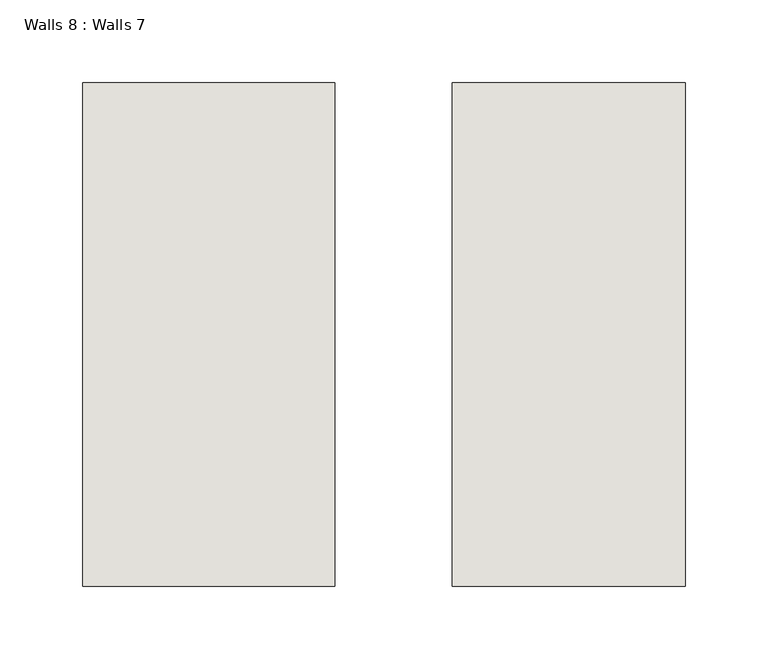
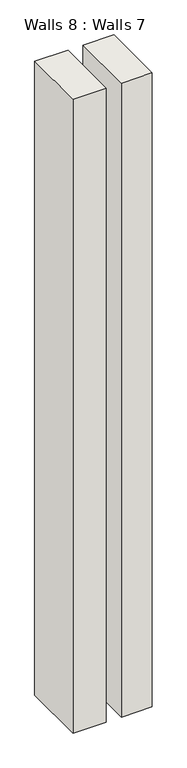
"""IFC4 building model written with IfcOpenShell, lengths in millimetres: wall geometry, Walls 8 : Walls 7."""

from ifc_helpers import new_model, si_unit, origin, origin_with_axes, place, context, project, spatial, polyline, outline, extrude, source, transform, mapped, element, save


def walls_8_walls_7_cfda60ff(model_context):
    return source(origin(), model_context, "Body", "SweptSolid", [
        extrude(outline(polyline([(-12329.6424966, 401.1257411), (-12329.6424966, 96.3257411), (-12482.0424966, 96.3257411), (-12482.0424966, 401.1257411), (-12329.6424966, 401.1257411)])), origin_with_axes(), (0.0, 0.0, 1.0), 3086.7795043),
        extrude(outline(polyline([(-12117.3437624, 401.1257411), (-12117.3437624, 96.3257411), (-12258.517466, 96.3257411), (-12258.517466, 401.1257411), (-12117.3437624, 401.1257411)])), origin_with_axes(), (0.0, 0.0, 1.0), 3086.7795043),
    ])


if __name__ == "__main__":
    model = new_model("IFC4")
    model_context = context("Model", 3, world=origin())
    ifc_project = project(units=[si_unit("LENGTHUNIT", "METRE", prefix="MILLI")], contexts=[model_context])
    site = spatial("IfcSite", under=ifc_project)
    building = spatial("IfcBuilding", under=site)
    placement = place(None, origin())
    walls_8_walls_7_shape = walls_8_walls_7_cfda60ff(model_context)
    element("IfcWall", 1, ObjectType="Walls 8 : Walls 7", at=placement, inside=building, context=model_context, shape_type="MappedRepresentation", body=[
        mapped(walls_8_walls_7_shape, transform((0.0, 0.0, 0.0), x_axis=(1.0, 0.0, 0.0), y_axis=(0.0, 1.0, 0.0), z_axis=(0.0, 0.0, 1.0))),
    ])
    save(model, "model.ifc")

# Revit data of these elements
# Element 1 (IfcWall, "Walls 8 : Walls 7")
#   Materials on its faces: "Default Wall"
# Materials
#   "Default Wall": colour RGB 128 128 128, transparency 0
